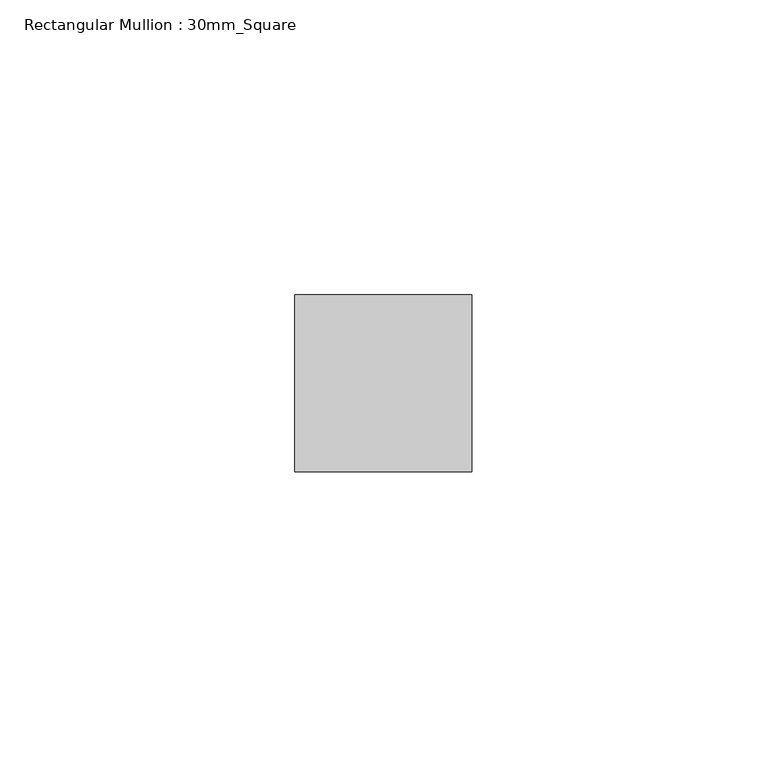
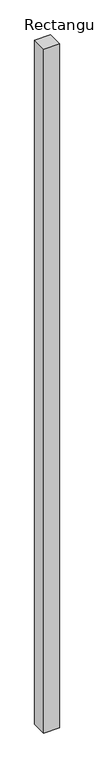
"""IFC4 building model written with IfcOpenShell, lengths in millimetres: member geometry, Rectangular Mullion : 30mm_Square."""

from ifc_helpers import new_model, si_unit, frame, origin, place, context, project, spatial, polyline, outline, extrude, source, transform, mapped, element, save


def rectangular_mullion_30mm_square_75078aee(model_context):
    return source(origin(), model_context, "Body", "SweptSolid", [
        extrude(outline(polyline([(0.0, 15.0), (0.0, -15.0), (-30.0, -15.0), (-30.0, 15.0), (0.0, 15.0)])), frame((0.0, 0.0, -1387.491145), z_axis=(0.0, 0.0, 1.0), x_axis=(1.0, 0.0, 0.0)), (0.0, 0.0, 1.0), 1387.491145),
    ])


if __name__ == "__main__":
    model = new_model("IFC4")
    model_context = context("Model", 3, world=origin())
    ifc_project = project(units=[si_unit("LENGTHUNIT", "METRE", prefix="MILLI")], contexts=[model_context])
    site = spatial("IfcSite", under=ifc_project)
    building = spatial("IfcBuilding", under=site)
    placement = place(None, origin())
    rectangular_mullion_30mm_square_shape = rectangular_mullion_30mm_square_75078aee(model_context)
    element("IfcMember", 1, ObjectType="Rectangular Mullion : 30mm_Square", at=placement, inside=building, context=model_context, shape_type="MappedRepresentation", body=[
        mapped(rectangular_mullion_30mm_square_shape, transform((0.0, 0.0, 0.0), x_axis=(1.0, 0.0, 0.0), y_axis=(0.0, 1.0, 0.0), z_axis=(0.0, 0.0, 1.0))),
    ])
    save(model, "model.ifc")

# Revit data of these elements
# Type "Rectangular Mullion : 30mm_Square"
#   Keynote = "H11"
#   built-in parameter 1007304 = 0.0984252 (stored number, unit not read)
#   built-in parameter 1007301 = 0.0492126 (stored number, unit not read)
#   built-in parameter 1007300 = 0.0492126 (stored number, unit not read)
# Element 1 (IfcMember, "Rectangular Mullion : 30mm_Square")
#   Materials on its faces: "Aluminium"
# Materials
#   "Aluminium": class "Metal", colour RGB 247 247 247, transparency 0, Description = "Aluminium 6061", Cost = 0
